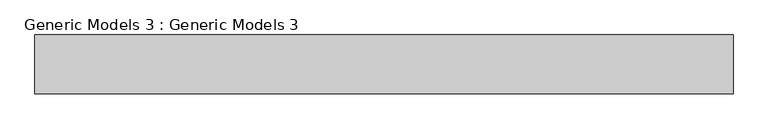
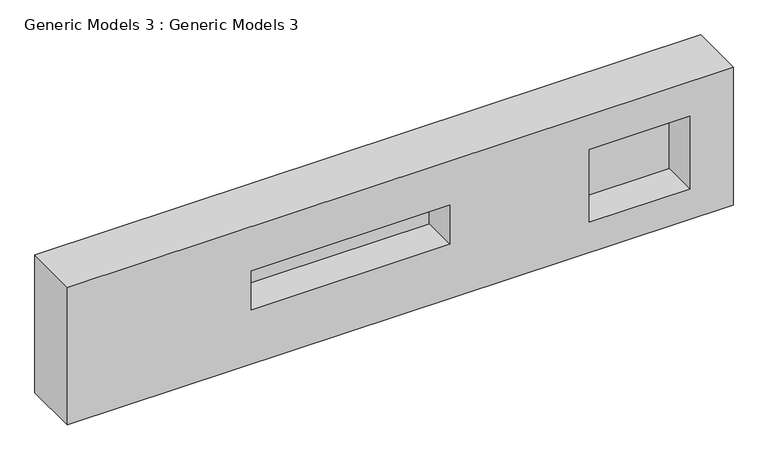
"""IFC4 building model written with IfcOpenShell, lengths in millimetres: proxy geometry, Generic Models 3 : Generic Models 3."""

from ifc_helpers import new_model, si_unit, origin, place, context, project, spatial, faceted_brep, source, transform, mapped, element, save


def generic_models_3_generic_models_3_4ea04a15(model_context):
    return source(origin(), model_context, "Body", "Brep", [
        faceted_brep([(-14536.2782619, -4597.9088252, 5913.3913732), (-20239.176744, -4597.9088252, 5913.3913732), (-20239.176744, -4597.9088252, 4664.6984502), (-14536.2782619, -4597.9088252, 4664.6984502), (-16963.8414406, -4597.9088252, 5157.3503387), (-18665.6414406, -4597.9088252, 5157.3503387), (-18665.6414406, -4597.9088252, 5511.8999235), (-16963.8414406, -4597.9088252, 5511.8999235), (-14907.0126903, -4597.9088252, 5599.46741), (-14907.0126903, -4597.9088252, 4939.06741), (-15770.6126903, -4597.9088252, 4939.06741), (-15770.6126903, -4597.9088252, 5599.46741), (-14536.2782619, -4115.9699953, 5913.3913732), (-14536.2782619, -4115.9699953, 4664.6984502), (-20239.176744, -4115.9699953, 4664.6984502), (-20239.176744, -4115.9699953, 5913.3913732), (-16963.8414406, -4293.1088252, 5157.3503387), (-18665.6414406, -4293.1088252, 5157.3503387), (-18665.6414406, -4293.1088252, 5511.8999235), (-16963.8414406, -4293.1088252, 5511.8999235), (-14907.0126903, -4293.1088252, 5599.46741), (-14907.0126903, -4293.1088252, 4939.06741), (-15770.6126903, -4293.1088252, 4939.06741), (-15770.6126903, -4293.1088252, 5599.46741)], [[[0, 1, 2, 3], [4, 5, 6, 7], [8, 9, 10, 11]], [[12, 13, 14, 15]], [[1, 0, 12, 15]], [[2, 1, 15, 14]], [[3, 2, 14, 13]], [[0, 3, 13, 12]], [[16, 17, 5, 4]], [[17, 18, 6, 5]], [[18, 19, 7, 6]], [[19, 16, 4, 7]], [[20, 21, 9, 8]], [[21, 22, 10, 9]], [[22, 23, 11, 10]], [[23, 20, 8, 11]], [[16, 19, 18, 17]], [[20, 23, 22, 21]]]),
    ])


if __name__ == "__main__":
    model = new_model("IFC4")
    model_context = context("Model", 3, world=origin())
    ifc_project = project(units=[si_unit("LENGTHUNIT", "METRE", prefix="MILLI")], contexts=[model_context])
    site = spatial("IfcSite", under=ifc_project)
    building = spatial("IfcBuilding", under=site)
    placement = place(None, origin())
    generic_models_3_generic_models_3_shape = generic_models_3_generic_models_3_4ea04a15(model_context)
    element("IfcBuildingElementProxy", 1, Name="Generic Models 3 : Generic Models 3", ObjectType="Generic Models 3 : Generic Models 3", at=placement, inside=building, context=model_context, shape_type="MappedRepresentation", body=[
        mapped(generic_models_3_generic_models_3_shape, transform((0.0, 0.0, 0.0), x_axis=(1.0, 0.0, 0.0), y_axis=(0.0, 1.0, 0.0), z_axis=(0.0, 0.0, 1.0))),
    ])
    save(model, "model.ifc")
